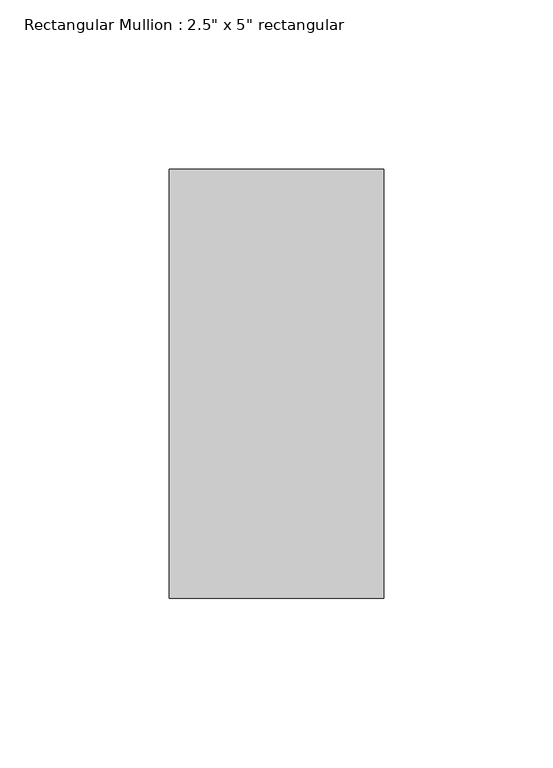
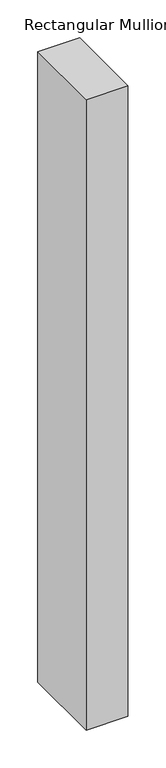
"""IFC4 building model written with IfcOpenShell, lengths in millimetres: member geometry."""

from ifc_helpers import new_model, si_unit, frame, origin, place, context, project, spatial, polyline, outline, extrude, source, transform, mapped, element, save


def member_fde90c6a(model_context):
    return source(origin(), model_context, "Body", "SweptSolid", [
        extrude(outline(polyline([(31.75, 63.5), (31.75, -63.5), (-31.75, -63.5), (-31.75, 63.5), (31.75, 63.5)])), frame((0.0, 0.0, -1013.8675922), z_axis=(0.0, 0.0, 1.0), x_axis=(1.0, 0.0, 0.0)), (0.0, 0.0, 1.0), 1013.8675922),
    ])


if __name__ == "__main__":
    model = new_model("IFC4")
    model_context = context("Model", 3, world=origin())
    ifc_project = project(units=[si_unit("LENGTHUNIT", "METRE", prefix="MILLI")], contexts=[model_context])
    site = spatial("IfcSite", under=ifc_project)
    building = spatial("IfcBuilding", under=site)
    placement = place(None, origin())
    member_shape = member_fde90c6a(model_context)
    element("IfcMember", 1, ObjectType="Rectangular Mullion : 2.5\" x 5\" rectangular", at=placement, inside=building, context=model_context, shape_type="MappedRepresentation", body=[
        mapped(member_shape, transform((0.0, 0.0, 0.0), x_axis=(1.0, 0.0, 0.0), y_axis=(0.0, 1.0, 0.0), z_axis=(0.0, 0.0, 1.0))),
    ])
    save(model, "model.ifc")

# Revit data of these elements
# Type "Rectangular Mullion : 2.5\" x 5\" rectangular"
#   built-in parameter 1007304 = 0.416667 (stored number, unit not read)
#   built-in parameter 1007301 = 0.104167 (stored number, unit not read)
#   built-in parameter 1007300 = 0.104167 (stored number, unit not read)
# Element 1 (IfcMember, "Rectangular Mullion : 2.5\" x 5\" rectangular")
#   Materials on its faces: "Aluminum"
# Materials
#   "Aluminum": class "Metal", colour RGB 247 247 247, transparency 0, Description = "Aluminum 6061", Cost = 0
